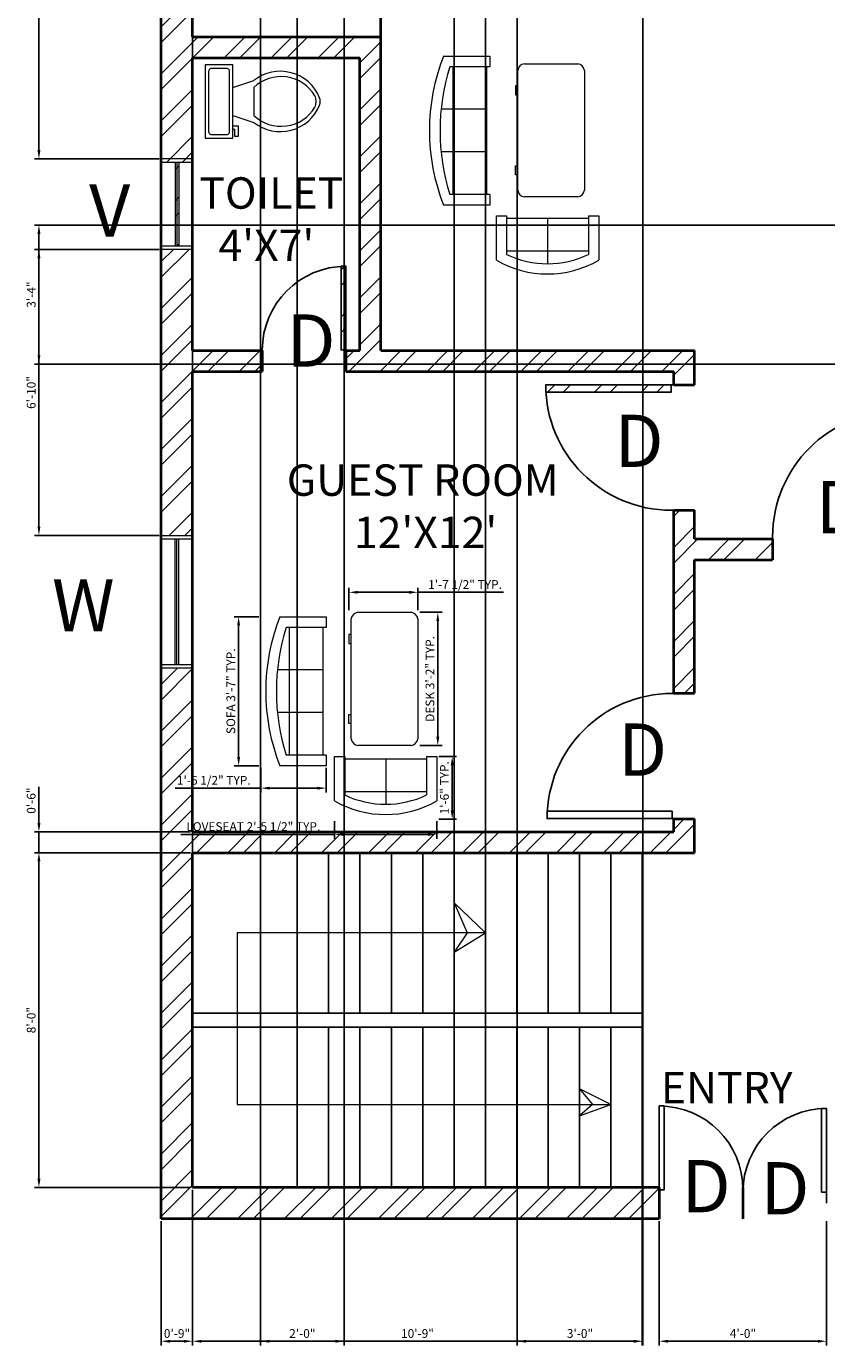
# Model space of a CAD drawing. Units: inches. Extents: x 1143 to 1626, y 7431 to 8140.
# Tile 1 of 4: x 1143 to 1373, y 7431 to 7809. Entities that reach past the tile are written whole.
import ezdxf

# ---------------------------------------------------------------- set-up
doc = ezdxf.new("R2010")
doc.units = ezdxf.units.IN
for name, color, linetype, lineweight in [('A-ANNO-DIMS', 4, 'Continuous', 18), ('A-ANNO-SYMB', 7, 'Continuous', 18), ('A-DOOR', 3, 'Continuous', 25), ('A-FLOR-STRS', 7, 'Continuous', 25), ('A-GLAZ', 4, 'Continuous', 18), ('A-WALL', 2, 'Continuous', 40), ('A-WALL-PATT', 7, 'Continuous', 13)]:
    doc.layers.add(name, color=color, linetype=linetype, lineweight=lineweight)
for name, color, linetype, lineweight, true_color in [('A-ANNO-TEXT', 40, 'Continuous', 18, 0xf8d731), ('A-AREA-IDEN', 40, 'Continuous', 25, 0xf8d731), ('A-FLOR-FIXT', 40, 'Continuous', 18, 0xf8d731), ('A-FURN', 40, 'Continuous', 18, 0xf8d731)]:
    doc.layers.add(name, color=color, linetype=linetype, lineweight=lineweight, true_color=true_color)
doc.styles.get("Standard").update_dxf_attribs({"font": 'arial.ttf'})
doc.dimstyles.new('ISO-25', dxfattribs={"dimtxt": 2.5, "dimasz": 2.5, "dimexe": 1.25, "dimexo": 0.625, "dimtad": 1, "dimdec": 0, "dimlunit": 3, "dimtxsty": 'Standard', "dimcen": 2.5, "dimadec": 0, "dimazin": 0, "dimtfac": 1, "dimtdec": 0, "dimtmove": 0, "dimatfit": 3, "dimfxl": 1, "dimarcsym": 0})

# ---------------------------------------------------------------- blocks, each defined once
blk = doc.blocks.new('*U8')
for p, q in [((0, 0), (0, -100)), ((750, 0), (750, -100))]:
    blk.add_line(p, q)
blk.add_lwpolyline([(0, 0), (0, 750), (43.75, 750), (43.75, 0)], close=True)
blk.add_arc((0, 0), 750, 0, 90)
blk = doc.blocks.new('Desk - 30 x 60 in.')
for p, q in [((-26.999995, 0), (26.999995, 0)), ((-29.999995, -27), (-29.999995, -3)), ((29.999995, -3), (29.999995, -27)), ((26.999995, -30), (-26.999995, -30)), ((-20.000005, -30), (-20.000005, -31)), ((-20.000005, -31), (-16.000005, -31)), ((-16.000005, -31), (-16.000005, -30)), ((15.999995, -31), (15.999995, -30)), ((19.999995, -31), (15.999995, -31)), ((19.999995, -30), (19.999995, -31))]:
    blk.add_line(p, q)
for centre, start, end in [((-26.499995, -3.5), 98.1301, 171.8699), ((26.499995, -3.5), 8.130102, 81.8699), ((-26.499995, -26.5), 188.1301, 261.8699), ((26.499995, -26.5), 278.1301, 351.8699)]:
    blk.add_arc(centre, 3.535534, start, end)
blk = doc.blocks.new('Sofa - Roundback 7 ft.')
for p, q in [((-12.00002, -32.4421), (-12.00003, -6.5971)), ((11.99997, -32.4421), (11.99998, -6.5971)), ((-36.000027, -34), (-36.000027, -11.4696)), ((-35.999844, -13.3819), (35.9998, -13.3819)), ((35.99998, -34), (35.99998, -11.4696)), ((-36.000027, -32.4421), (35.99998, -32.4421))]:
    blk.add_line(p, q)
for points in [[(-36.000027, -34), (-42.000027, -34), (-42.000027, -8)], [(41.99998, -8), (41.99998, -34), (35.99998, -34)]]:
    blk.add_lwpolyline(points)
for centre, radius, start, end in [((0, -114.25), 114.25, 68.43141, 111.5686), ((-0.00001, -127.1968), 121.1968, 72.72033, 107.2797)]:
    blk.add_arc(centre, radius, start, end)
blk = doc.blocks.new('Sofa - Roundback Loveseat 5 ft.')
for p, q in [((0, -32.44198), (0, -5.99998)), ((-24, -33.99998), (-24, -11.46958)), ((-23.9998, -13.38178), (23.99986, -13.38178)), ((24.00004, -33.99998), (24.00004, -11.46958)), ((-24, -32.44198), (24.00004, -32.44198))]:
    blk.add_line(p, q)
for points in [[(-24, -33.99998), (-30, -33.99998), (-30, -7.99998)], [(30.00004, -7.99998), (30.00004, -33.99998), (24.00004, -33.99998)]]:
    blk.add_lwpolyline(points)
for centre, radius, start, end in [((0, -60.24998), 60.24998, 60.13715, 119.8628), ((0, -61.38438), 55.38444, 64.32083, 115.6792)]:
    blk.add_arc(centre, radius, start, end)
blk = doc.blocks.new('Toilet - top')
for p, q in [((9.5, -6), (9.5, -2)), ((-10, -8.5), (-8, -8.5)), ((-10, -9.5), (-10, -8.5)), ((-7, -9.5), (-10, -9.5)), ((-8, -8.5), (-8, -8)), ((-7, -8), (-7, -9.5)), ((-4, -8), (-6, -14)), ((4, -8), (6, -14)), ((4, -14), (-4, -14))]:
    blk.add_line(p, q)
blk.add_lwpolyline([(10.5, -8), (10.5, 0), (-10.5, 0), (-10.5, -8)], close=True)
for points in [[(-9.5, -2), (-9.5, -6)], [(8.5, -1), (-8.5, -1)], [(-8.5, -7), (8.5, -7)]]:
    blk.add_lwpolyline(points)
for centre, radius, start, end in [((-8.62, -1.88), 0.884, 81.8699, 188.1301), ((8.62, -1.88), 0.884, 351.8699, 98.1301), ((-8.62, -6.12), 0.884, 171.8699, 278.1301), ((8.62, -6.12), 0.884, 261.8699, 8.1301), ((3.52, -21.58), 12.17, 141.4691, 247.9714), ((4.2, -21.82), 11.33, 136.3677, 238.9468), ((-3.52, -21.58), 12.17, 292.0284, 38.5307), ((-4.2, -21.82), 11.33, 301.053, 43.6321), ((0, -27.88), 4, 245.7318, 294.2682), ((0, -29), 4, 254.8605, 285.1395)]:
    blk.add_arc(centre, radius, start, end)
blk = doc.blocks.new('WIN-36IN')
for p, q in [((0, 9), (0, 0)), ((1, 9), (1, 0)), ((37, 9), (37, 0)), ((38, 9), (38, 0)), ((1, 5), (37, 5)), ((1, 4.5), (37, 4.5)), ((1, 4), (37, 4))]:
    blk.add_line(p, q)
blk = doc.blocks.new('WIN-24IN')
for p, q in [((0, 9), (0, 0)), ((1, 9), (1, 0)), ((25, 9), (25, 0)), ((26, 9), (26, 0)), ((1, 5), (25, 5)), ((1, 4.5), (25, 4.5)), ((1, 4), (25, 4))]:
    blk.add_line(p, q)
blk = doc.blocks.new('*D70')
at = {"layer": 'A-ANNO-DIMS', "color": 0, "lineweight": -2, "transparency": 16777216}
for p, q in [((1256.06, 7641.36), (1262.42, 7641.36)), ((1261.17, 7638.86), (1261.17, 7605.65)), ((1256.06, 7603.15), (1262.42, 7603.15))]:
    blk.add_line(p, q, dxfattribs=at)
at = {"layer": 'A-ANNO-DIMS', "color": 0, "transparency": 16777216}
for points in [[(1260.75, 7638.86), (1261.59, 7638.86), (1261.17, 7641.36)], [(1260.75, 7605.65), (1261.59, 7605.65), (1261.17, 7603.15)]]:
    blk.add_solid(points, dxfattribs=at)
at = {"layer": 'Defpoints', "color": 0, "transparency": 16777216}
for p in [(1255.44, 7641.36), (1255.44, 7603.15), (1261.17, 7603.15)]:
    blk.add_point(p, dxfattribs=at)
at = {"layer": 'A-ANNO-DIMS', "color": 0, "transparency": 16777216, "insert": (1259.25, 7622.25), "char_height": 2.5, "attachment_point": 5, "rotation": 90}
blk.add_mtext('DESK 3\'-2" TYP.', dxfattribs=at)
blk = doc.blocks.new('*D71')
at = {"layer": 'A-ANNO-DIMS', "color": 0, "lineweight": -2, "transparency": 16777216}
for p, q in [((1235.7, 7641.99), (1235.7, 7648.34)), ((1238.2, 7647.09), (1252.94, 7647.09)), ((1255.44, 7641.99), (1255.44, 7648.34)), ((1255.44, 7647.09), (1280.02, 7647.09))]:
    blk.add_line(p, q, dxfattribs=at)
at = {"layer": 'A-ANNO-DIMS', "color": 0, "transparency": 16777216}
for points in [[(1238.2, 7647.51), (1238.2, 7646.68), (1235.7, 7647.09)], [(1252.94, 7647.51), (1252.94, 7646.68), (1255.44, 7647.09)]]:
    blk.add_solid(points, dxfattribs=at)
at = {"layer": 'Defpoints', "color": 0, "transparency": 16777216}
for p in [(1255.44, 7647.09), (1235.7, 7641.36), (1255.44, 7641.36)]:
    blk.add_point(p, dxfattribs=at)
at = {"layer": 'A-ANNO-DIMS', "color": 0, "transparency": 16777216, "insert": (1268.98, 7649.01), "char_height": 2.5, "attachment_point": 5}
blk.add_mtext('1\'-7 1/2" TYP.', dxfattribs=at)
blk = doc.blocks.new('*D72')
at = {"layer": 'A-ANNO-DIMS', "color": 0, "lineweight": -2, "transparency": 16777216}
for p, q in [((1209.82, 7640.1), (1202.79, 7640.1)), ((1204.04, 7599.84), (1204.04, 7637.6)), ((1209.82, 7597.34), (1202.79, 7597.34))]:
    blk.add_line(p, q, dxfattribs=at)
at = {"layer": 'A-ANNO-DIMS', "color": 0, "transparency": 16777216}
for points in [[(1203.62, 7637.6), (1204.45, 7637.6), (1204.04, 7640.1)], [(1203.62, 7599.84), (1204.45, 7599.84), (1204.04, 7597.34)]]:
    blk.add_solid(points, dxfattribs=at)
at = {"layer": 'Defpoints', "color": 0, "transparency": 16777216}
for p in [(1204.04, 7640.1), (1210.45, 7640.1), (1210.45, 7597.34)]:
    blk.add_point(p, dxfattribs=at)
at = {"layer": 'A-ANNO-DIMS', "color": 0, "transparency": 16777216, "insert": (1202.12, 7618.72), "char_height": 2.5, "attachment_point": 5, "rotation": 90}
blk.add_mtext('SOFA 3\'-7" TYP.', dxfattribs=at)
blk = doc.blocks.new('*D73')
at = {"layer": 'A-ANNO-DIMS', "color": 0, "lineweight": -2, "transparency": 16777216}
for p, q in [((1210.45, 7596.72), (1210.45, 7589.68)), ((1229.11, 7596.72), (1229.11, 7589.68)), ((1210.45, 7590.93), (1185.87, 7590.93)), ((1226.61, 7590.93), (1212.95, 7590.93))]:
    blk.add_line(p, q, dxfattribs=at)
at = {"layer": 'A-ANNO-DIMS', "color": 0, "transparency": 16777216}
for points in [[(1212.95, 7591.34), (1212.95, 7590.51), (1210.45, 7590.93)], [(1226.61, 7591.34), (1226.61, 7590.51), (1229.11, 7590.93)]]:
    blk.add_solid(points, dxfattribs=at)
at = {"layer": 'Defpoints', "color": 0, "transparency": 16777216}
for p in [(1210.45, 7597.34), (1229.11, 7597.34), (1210.45, 7590.93)]:
    blk.add_point(p, dxfattribs=at)
at = {"layer": 'A-ANNO-DIMS', "color": 0, "transparency": 16777216, "insert": (1196.91, 7592.85), "char_height": 2.5, "attachment_point": 5}
blk.add_mtext('1\'-6 1/2" TYP.', dxfattribs=at)
blk = doc.blocks.new('*D74')
at = {"layer": 'A-ANNO-DIMS', "color": 0, "lineweight": -2, "transparency": 16777216}
for p, q in [((1231.54, 7581.44), (1231.54, 7576.41)), ((1260.9, 7581.44), (1260.9, 7576.41)), ((1231.54, 7577.66), (1187.43, 7577.66)), ((1258.4, 7577.66), (1234.04, 7577.66))]:
    blk.add_line(p, q, dxfattribs=at)
at = {"layer": 'A-ANNO-DIMS', "color": 0, "transparency": 16777216}
for points in [[(1234.04, 7578.07), (1234.04, 7577.24), (1231.54, 7577.66)], [(1258.4, 7578.07), (1258.4, 7577.24), (1260.9, 7577.66)]]:
    blk.add_solid(points, dxfattribs=at)
at = {"layer": 'Defpoints', "color": 0, "transparency": 16777216}
for p in [(1231.54, 7582.06), (1260.9, 7582.06), (1231.54, 7577.66)]:
    blk.add_point(p, dxfattribs=at)
at = {"layer": 'A-ANNO-DIMS', "color": 0, "transparency": 16777216, "insert": (1208.24, 7579.58), "char_height": 2.5, "attachment_point": 5}
blk.add_mtext('LOVESEAT 2\'-5 1/2" TYP.', dxfattribs=at)
blk = doc.blocks.new('*D75')
at = {"layer": 'A-ANNO-DIMS', "color": 0, "lineweight": -2, "transparency": 16777216}
for p, q in [((1261.52, 7600), (1266.55, 7600)), ((1265.3, 7597.5), (1265.3, 7584.56)), ((1261.52, 7582.06), (1266.55, 7582.06))]:
    blk.add_line(p, q, dxfattribs=at)
at = {"layer": 'A-ANNO-DIMS', "color": 0, "transparency": 16777216}
for points in [[(1264.89, 7597.5), (1265.72, 7597.5), (1265.3, 7600)], [(1264.89, 7584.56), (1265.72, 7584.56), (1265.3, 7582.06)]]:
    blk.add_solid(points, dxfattribs=at)
at = {"layer": 'Defpoints', "color": 0, "transparency": 16777216}
for p in [(1260.9, 7600), (1260.9, 7582.06), (1265.3, 7582.06)]:
    blk.add_point(p, dxfattribs=at)
at = {"layer": 'A-ANNO-DIMS', "color": 0, "transparency": 16777216, "insert": (1263.4, 7591.03), "char_height": 2.5, "attachment_point": 5, "rotation": 90}
blk.add_mtext('1\'-6" TYP.', dxfattribs=at)
blk = doc.blocks.new('*D80')
at = {"layer": 'A-ANNO-DIMS', "color": 0, "lineweight": -2, "transparency": 16777216}
for p, q in [((1190.85, 7475.77), (1190.85, 7431.05)), ((1319.85, 7475.77), (1319.85, 7431.05)), ((1193.35, 7432.3), (1317.35, 7432.3))]:
    blk.add_line(p, q, dxfattribs=at)
at = {"layer": 'A-ANNO-DIMS', "color": 0, "transparency": 16777216}
for points in [[(1193.35, 7432.71), (1193.35, 7431.88), (1190.85, 7432.3)], [(1317.35, 7432.71), (1317.35, 7431.88), (1319.85, 7432.3)]]:
    blk.add_solid(points, dxfattribs=at)
at = {"layer": 'Defpoints', "color": 0, "transparency": 16777216}
for p in [(1190.85, 7476.4), (1319.85, 7476.4), (1319.85, 7432.3)]:
    blk.add_point(p, dxfattribs=at)
at = {"layer": 'A-ANNO-DIMS', "color": 0, "transparency": 16777216, "insert": (1255.35, 7434.2), "char_height": 2.5, "attachment_point": 5}
blk.add_mtext('10\'-9"', dxfattribs=at)
blk = doc.blocks.new('*D81')
at = {"layer": 'A-ANNO-DIMS', "color": 0, "lineweight": -2, "transparency": 16777216}
for p, q in [((1190.23, 7572.4), (1145.5, 7572.4)), ((1146.75, 7478.9), (1146.75, 7569.9)), ((1190.23, 7476.4), (1145.5, 7476.4))]:
    blk.add_line(p, q, dxfattribs=at)
at = {"layer": 'A-ANNO-DIMS', "color": 0, "transparency": 16777216}
for points in [[(1146.33, 7569.9), (1147.17, 7569.9), (1146.75, 7572.4)], [(1146.33, 7478.9), (1147.17, 7478.9), (1146.75, 7476.4)]]:
    blk.add_solid(points, dxfattribs=at)
at = {"layer": 'Defpoints', "color": 0, "transparency": 16777216}
for p in [(1146.75, 7572.4), (1190.85, 7572.4), (1190.85, 7476.4)]:
    blk.add_point(p, dxfattribs=at)
at = {"layer": 'A-ANNO-DIMS', "color": 0, "transparency": 16777216, "insert": (1144.85, 7524.4), "char_height": 2.5, "attachment_point": 5, "rotation": 90}
blk.add_mtext('8\'-0"', dxfattribs=at)
blk = doc.blocks.new('*D82')
at = {"layer": 'A-ANNO-DIMS', "color": 0, "lineweight": -2, "transparency": 16777216}
for p, q in [((1324.72, 7466.77), (1324.72, 7431.05)), ((1372.72, 7466.77), (1372.72, 7431.05)), ((1327.22, 7432.3), (1370.22, 7432.3))]:
    blk.add_line(p, q, dxfattribs=at)
at = {"layer": 'A-ANNO-DIMS', "color": 0, "transparency": 16777216}
for points in [[(1327.22, 7432.71), (1327.22, 7431.88), (1324.72, 7432.3)], [(1370.22, 7432.71), (1370.22, 7431.88), (1372.72, 7432.3)]]:
    blk.add_solid(points, dxfattribs=at)
at = {"layer": 'Defpoints', "color": 0, "transparency": 16777216}
for p in [(1324.72, 7467.4), (1372.72, 7467.4), (1372.72, 7432.3)]:
    blk.add_point(p, dxfattribs=at)
at = {"layer": 'A-ANNO-DIMS', "color": 0, "transparency": 16777216, "insert": (1348.72, 7434.2), "char_height": 2.5, "attachment_point": 5}
blk.add_mtext('4\'-0"', dxfattribs=at)
blk = doc.blocks.new('*D83')
at = {"layer": 'A-ANNO-DIMS', "color": 0, "lineweight": -2, "transparency": 16777216}
for p, q in [((1190.85, 7475.77), (1190.85, 7431.05)), ((1181.85, 7466.77), (1181.85, 7431.05)), ((1184.35, 7432.3), (1188.35, 7432.3))]:
    blk.add_line(p, q, dxfattribs=at)
at = {"layer": 'A-ANNO-DIMS', "color": 0, "transparency": 16777216}
for points in [[(1184.35, 7432.71), (1184.35, 7431.88), (1181.85, 7432.3)], [(1188.35, 7432.71), (1188.35, 7431.88), (1190.85, 7432.3)]]:
    blk.add_solid(points, dxfattribs=at)
at = {"layer": 'Defpoints', "color": 0, "transparency": 16777216}
for p in [(1190.85, 7476.4), (1181.85, 7467.4), (1190.85, 7432.3)]:
    blk.add_point(p, dxfattribs=at)
at = {"layer": 'A-ANNO-DIMS', "color": 0, "transparency": 16777216, "insert": (1186.35, 7434.2), "char_height": 2.5, "attachment_point": 5}
blk.add_mtext('0\'-9"', dxfattribs=at)
blk = doc.blocks.new('*D84')
at = {"layer": 'A-ANNO-DIMS', "color": 0, "lineweight": -2, "transparency": 16777216}
for p, q in [((1146.75, 7580.9), (1146.75, 7591.29)), ((1190.23, 7578.4), (1145.5, 7578.4)), ((1146.75, 7572.4), (1146.75, 7578.4)), ((1190.23, 7572.4), (1145.5, 7572.4)), ((1146.75, 7569.9), (1146.75, 7567.4))]:
    blk.add_line(p, q, dxfattribs=at)
at = {"layer": 'A-ANNO-DIMS', "color": 0, "transparency": 16777216}
for points in [[(1146.33, 7580.9), (1147.17, 7580.9), (1146.75, 7578.4)], [(1146.33, 7569.9), (1147.17, 7569.9), (1146.75, 7572.4)]]:
    blk.add_solid(points, dxfattribs=at)
at = {"layer": 'Defpoints', "color": 0, "transparency": 16777216}
for p in [(1146.75, 7578.4), (1190.85, 7578.4), (1190.85, 7572.4)]:
    blk.add_point(p, dxfattribs=at)
at = {"layer": 'A-ANNO-DIMS', "color": 0, "transparency": 16777216, "insert": (1144.85, 7587.34), "char_height": 2.5, "attachment_point": 5, "rotation": 90}
blk.add_mtext('0\'-6"', dxfattribs=at)
blk = doc.blocks.new('*D85')
at = {"layer": 'A-ANNO-DIMS', "color": 0, "lineweight": -2, "transparency": 16777216}
for p, q in [((1283.96, 7931.77), (1283.96, 7431.05)), ((1319.96, 7931.77), (1319.96, 7431.05)), ((1286.46, 7432.3), (1317.46, 7432.3))]:
    blk.add_line(p, q, dxfattribs=at)
at = {"layer": 'A-ANNO-DIMS', "color": 0, "transparency": 16777216}
for points in [[(1286.46, 7432.71), (1286.46, 7431.88), (1283.96, 7432.3)], [(1317.46, 7432.71), (1317.46, 7431.88), (1319.96, 7432.3)]]:
    blk.add_solid(points, dxfattribs=at)
at = {"layer": 'Defpoints', "color": 0, "transparency": 16777216}
for p in [(1283.96, 7932.4), (1319.96, 7932.4), (1319.96, 7432.3)]:
    blk.add_point(p, dxfattribs=at)
at = {"layer": 'A-ANNO-DIMS', "color": 0, "transparency": 16777216, "insert": (1301.96, 7434.2), "char_height": 2.5, "attachment_point": 5}
blk.add_mtext('3\'-0"', dxfattribs=at)
blk = doc.blocks.new('*D86')
at = {"layer": 'A-ANNO-DIMS', "color": 0, "lineweight": -2, "transparency": 16777216}
for p, q in [((1210.31, 7841.77), (1210.31, 7431.05)), ((1234.31, 7841.77), (1234.31, 7431.05)), ((1212.81, 7432.3), (1231.81, 7432.3))]:
    blk.add_line(p, q, dxfattribs=at)
at = {"layer": 'A-ANNO-DIMS', "color": 0, "transparency": 16777216}
for points in [[(1212.81, 7432.71), (1212.81, 7431.88), (1210.31, 7432.3)], [(1231.81, 7432.71), (1231.81, 7431.88), (1234.31, 7432.3)]]:
    blk.add_solid(points, dxfattribs=at)
at = {"layer": 'Defpoints', "color": 0, "transparency": 16777216}
for p in [(1210.31, 7842.4), (1234.31, 7842.4), (1234.31, 7432.3)]:
    blk.add_point(p, dxfattribs=at)
at = {"layer": 'A-ANNO-DIMS', "color": 0, "transparency": 16777216, "insert": (1222.31, 7434.2), "char_height": 2.5, "attachment_point": 5}
blk.add_mtext('2\'-0"', dxfattribs=at)
blk = doc.blocks.new('*D91')
at = {"layer": 'A-ANNO-DIMS', "color": 0, "lineweight": -2, "transparency": 16777216}
for p, q in [((1181.23, 7745.4), (1145.5, 7745.4)), ((1146.75, 7665.9), (1146.75, 7742.9)), ((1181.23, 7663.4), (1145.5, 7663.4))]:
    blk.add_line(p, q, dxfattribs=at)
at = {"layer": 'A-ANNO-DIMS', "color": 0, "transparency": 16777216}
for points in [[(1146.33, 7742.9), (1147.17, 7742.9), (1146.75, 7745.4)], [(1146.33, 7665.9), (1147.17, 7665.9), (1146.75, 7663.4)]]:
    blk.add_solid(points, dxfattribs=at)
at = {"layer": 'Defpoints', "color": 0, "transparency": 16777216}
for p in [(1146.75, 7745.4), (1181.85, 7745.4), (1181.85, 7663.4)]:
    blk.add_point(p, dxfattribs=at)
at = {"layer": 'A-ANNO-DIMS', "color": 0, "transparency": 16777216, "insert": (1144.85, 7704.4), "char_height": 2.5, "attachment_point": 5, "rotation": 90}
blk.add_mtext('6\'-10"', dxfattribs=at)
blk = doc.blocks.new('*D92')
at = {"layer": 'A-ANNO-DIMS', "color": 0, "lineweight": -2, "transparency": 16777216}
for p, q in [((1181.23, 7877.4), (1145.5, 7877.4)), ((1146.75, 7773.9), (1146.75, 7874.9)), ((1181.23, 7771.4), (1145.5, 7771.4))]:
    blk.add_line(p, q, dxfattribs=at)
at = {"layer": 'A-ANNO-DIMS', "color": 0, "transparency": 16777216}
for points in [[(1146.33, 7874.9), (1147.17, 7874.9), (1146.75, 7877.4)], [(1146.33, 7773.9), (1147.17, 7773.9), (1146.75, 7771.4)]]:
    blk.add_solid(points, dxfattribs=at)
at = {"layer": 'Defpoints', "color": 0, "transparency": 16777216}
for p in [(1146.75, 7877.4), (1181.85, 7877.4), (1181.85, 7771.4)]:
    blk.add_point(p, dxfattribs=at)
at = {"layer": 'A-ANNO-DIMS', "color": 0, "transparency": 16777216, "insert": (1144.85, 7824.4), "char_height": 2.5, "attachment_point": 5, "rotation": 90}
blk.add_mtext('8\'-10"', dxfattribs=at)
blk = doc.blocks.new('*D98')
at = {"layer": 'A-ANNO-DIMS', "color": 0, "lineweight": -2, "transparency": 16777216}
for p, q in [((1190.85, 7477.02), (1190.85, 8103.75)), ((1193.35, 8102.5), (1218.35, 8102.5)), ((1220.85, 7477.02), (1220.85, 8103.75))]:
    blk.add_line(p, q, dxfattribs=at)
at = {"layer": 'A-ANNO-DIMS', "color": 0, "transparency": 16777216}
for points in [[(1193.35, 8102.91), (1193.35, 8102.08), (1190.85, 8102.5)], [(1218.35, 8102.91), (1218.35, 8102.08), (1220.85, 8102.5)]]:
    blk.add_solid(points, dxfattribs=at)
at = {"layer": 'Defpoints', "color": 0, "transparency": 16777216}
for p in [(1220.85, 8102.5), (1190.85, 7476.4), (1220.85, 7476.4)]:
    blk.add_point(p, dxfattribs=at)
at = {"layer": 'A-ANNO-DIMS', "color": 0, "transparency": 16777216, "insert": (1205.85, 8104.4), "char_height": 2.5, "attachment_point": 5}
blk.add_mtext('2\'-6"', dxfattribs=at)
blk = doc.blocks.new('*D99')
at = {"layer": 'A-ANNO-DIMS', "color": 0, "lineweight": -2, "transparency": 16777216}
for p, q in [((1265.85, 7477.02), (1265.85, 8103.75)), ((1268.35, 8102.5), (1272.35, 8102.5)), ((1274.85, 7477.02), (1274.85, 8103.75))]:
    blk.add_line(p, q, dxfattribs=at)
at = {"layer": 'A-ANNO-DIMS', "color": 0, "transparency": 16777216}
for points in [[(1268.35, 8102.91), (1268.35, 8102.08), (1265.85, 8102.5)], [(1272.35, 8102.91), (1272.35, 8102.08), (1274.85, 8102.5)]]:
    blk.add_solid(points, dxfattribs=at)
at = {"layer": 'Defpoints', "color": 0, "transparency": 16777216}
for p in [(1274.85, 8102.5), (1265.85, 7476.4), (1274.85, 7476.4)]:
    blk.add_point(p, dxfattribs=at)
at = {"layer": 'A-ANNO-DIMS', "color": 0, "transparency": 16777216, "insert": (1270.35, 8104.4), "char_height": 2.5, "attachment_point": 5}
blk.add_mtext('0\'-9"', dxfattribs=at)
blk = doc.blocks.new('*D103')
at = {"layer": 'A-ANNO-DIMS', "color": 0, "lineweight": -2, "transparency": 16777216}
for p, q in [((1430.23, 7752.4), (1145.5, 7752.4)), ((1146.75, 7715.06), (1146.75, 7749.9)), ((1430.23, 7712.56), (1145.5, 7712.56))]:
    blk.add_line(p, q, dxfattribs=at)
at = {"layer": 'A-ANNO-DIMS', "color": 0, "transparency": 16777216}
for points in [[(1146.33, 7749.9), (1147.17, 7749.9), (1146.75, 7752.4)], [(1146.33, 7715.06), (1147.17, 7715.06), (1146.75, 7712.56)]]:
    blk.add_solid(points, dxfattribs=at)
at = {"layer": 'Defpoints', "color": 0, "transparency": 16777216}
for p in [(1146.75, 7752.4), (1430.85, 7752.4), (1430.85, 7712.56)]:
    blk.add_point(p, dxfattribs=at)
at = {"layer": 'A-ANNO-DIMS', "color": 0, "transparency": 16777216, "insert": (1144.85, 7732.48), "char_height": 2.5, "attachment_point": 5, "rotation": 90}
blk.add_mtext('3\'-4"', dxfattribs=at)

msp = doc.modelspace()

# ---------------------------------------------------------------- hatches: boundary and pattern name
at = {"layer": 'A-WALL-PATT'}
h = msp.add_hatch(dxfattribs=at)
h.set_pattern_fill('ANSI32', color=256)
h.paths.add_polyline_path([(1240.85, 8067.4), (1181.85, 8067.4), (1181.85, 8017.4), (1190.85, 8017.4), (1190.85, 8058.4), (1240.85, 8058.4)])
h.paths.add_polyline_path([(1541.85, 8067.4), (1486.85, 8067.4), (1486.85, 8058.4), (1532.85, 8058.4), (1532.85, 8017.4), (1541.85, 8017.4)], flags=17)
h.paths.add_polyline_path([(1352.85, 8067.4), (1278.85, 8067.4), (1278.85, 8058.4), (1328.85, 8058.4), (1328.85, 7938.4), (1319.96, 7938.4), (1319.96, 7932.4), (1334.85, 7932.4), (1334.85, 7956.4), (1338.11, 7956.4), (1338.11, 7962.4), (1334.85, 7962.4), (1334.85, 8010.4), (1396.85, 8010.4), (1396.85, 7962.4), (1386.11, 7962.4), (1386.11, 7956.4), (1396.85, 7956.4), (1396.85, 7662.4), (1393.24, 7662.4), (1393.24, 7656.4), (1404.17, 7656.4), (1404.17, 7662.4), (1402.85, 7662.4), (1402.85, 7806.4), (1430.85, 7806.4), (1430.85, 7786.73), (1436.85, 7786.73), (1436.85, 7806.4), (1532.85, 7806.4), (1532.85, 7795.4), (1541.85, 7795.4), (1541.85, 7853.4), (1532.85, 7853.4), (1532.85, 7812.4), (1402.85, 7812.4), (1402.85, 7932.4), (1419.12, 7932.4), (1419.12, 7938.4), (1402.85, 7938.4), (1402.85, 8058.4), (1448.85, 8058.4), (1448.85, 8067.4), (1378.85, 8067.4), (1378.85, 8058.4), (1396.85, 8058.4), (1396.85, 8016.4), (1334.85, 8016.4), (1334.85, 8058.4), (1352.85, 8058.4)])
h.paths.add_polyline_path([(1283.96, 7938.4), (1190.85, 7938.4), (1190.85, 7979.4), (1181.85, 7979.4), (1181.85, 7903.4), (1190.85, 7903.4), (1190.85, 7932.4), (1238.85, 7932.4), (1238.85, 7848.4), (1234.31, 7848.4), (1234.31, 7842.4), (1244.85, 7842.4), (1244.85, 7932.4), (1283.96, 7932.4)])
h.paths.add_polyline_path([(1541.85, 7979.4), (1532.85, 7979.4), (1532.85, 7938.4), (1455.12, 7938.4), (1455.12, 7932.4), (1532.85, 7932.4), (1532.85, 7891.4), (1541.85, 7891.4)], flags=17)
h.paths.add_polyline_path([(1210.81, 7716.4), (1190.85, 7716.4), (1190.85, 7745.4), (1181.85, 7745.4), (1181.85, 7663.4), (1190.85, 7663.4), (1190.85, 7710.4), (1210.81, 7710.4)])
h.paths.add_polyline_path([(1232.89, 7871.85), (1232.89, 7871.89), (1234.29, 7871.89), (1234.29, 7847.89), (1232.89, 7847.89), (1232.89, 7871.85, 0.385662), (1210.31, 7848.85), (1210.31, 7842.4), (1190.85, 7842.4), (1190.85, 7806.4), (1244.85, 7806.4), (1244.85, 7716.4), (1325.66, 7716.4), (1334.85, 7716.4), (1334.85, 7706.63), (1328.13, 7706.63), (1328.13, 7704.53), (1292.13, 7704.53), (1292.13, 7706.63), (1328.85, 7706.63), (1328.85, 7710.4), (1325.66, 7710.4), (1234.81, 7710.4), (1234.81, 7716.6), (1233.41, 7716.6), (1233.41, 7740.6), (1234.81, 7740.6), (1234.81, 7716.4), (1238.85, 7716.4), (1238.85, 7800.4), (1190.85, 7800.4), (1190.85, 7770.4), (1186.85, 7770.4), (1186.85, 7746.4), (1185.85, 7746.4), (1185.85, 7770.4), (1181.85, 7770.4), (1181.85, 7878.4), (1190.85, 7878.4), (1190.85, 7848.4), (1210.3, 7848.4, -0.391105)])
h.paths.add_polyline_path([(1541.85, 7688.4), (1532.85, 7688.4), (1532.85, 7662.4), (1436.85, 7662.4), (1436.85, 7712.56), (1430.85, 7712.56), (1430.85, 7662.4), (1429.38, 7656.4), (1532.85, 7656.4), (1532.85, 7467.4), (1541.85, 7467.4)])
h.paths.add_polyline_path([(1334.85, 7656.4), (1357.24, 7656.4), (1357.24, 7662.4), (1334.85, 7662.4), (1334.85, 7670.63), (1328.85, 7670.63), (1328.85, 7618.14), (1334.85, 7618.14)])
h.paths.add_polyline_path([(1190.85, 7572.4), (1334.85, 7572.4), (1334.85, 7582.14), (1328.85, 7582.14), (1328.85, 7578.4), (1190.85, 7578.4), (1190.85, 7625.4), (1181.85, 7625.4), (1181.85, 7467.4), (1324.72, 7467.4), (1324.72, 7476.4), (1190.85, 7476.4)])

# ---------------------------------------------------------------- linework, layer by layer
at = {"layer": 'A-ANNO-SYMB'}
for p, q in [((1274.85, 7549.4), (1265.85, 7558.02)), ((1265.85, 7558.02), (1269.59, 7549.4)), ((1274.85, 7549.4), (1203.59, 7549.4)), ((1203.59, 7549.4), (1203.59, 7500.17)), ((1269.59, 7549.4), (1265.85, 7543.91)), ((1265.85, 7543.91), (1274.85, 7549.4)), ((1310.85, 7500.17), (1301.85, 7504.67)), ((1301.85, 7504.67), (1305.59, 7500.17)), ((1203.59, 7500.17), (1310.85, 7500.17)), ((1305.59, 7500.17), (1301.85, 7496.99)), ((1301.85, 7496.99), (1310.85, 7500.17))]:
    msp.add_line(p, q, dxfattribs=at)
at = {"layer": 'A-FLOR-STRS'}
for p, q in [((1220.85, 7476.4), (1220.85, 7572.4)), ((1229.85, 7526.4), (1229.85, 7572.4)), ((1238.85, 7526.4), (1238.85, 7572.4)), ((1247.85, 7526.4), (1247.85, 7572.4)), ((1256.85, 7526.4), (1256.85, 7572.4)), ((1265.85, 7526.4), (1265.85, 7572.4)), ((1274.85, 7526.4), (1274.85, 7572.4)), ((1283.85, 7526.4), (1283.85, 7572.4)), ((1292.85, 7526.4), (1292.85, 7572.4)), ((1301.85, 7526.4), (1301.85, 7572.4)), ((1301.85, 7526.4), (1301.85, 7572.4)), ((1310.85, 7526.4), (1310.85, 7572.4)), ((1319.85, 7476.4), (1319.85, 7572.4)), ((1319.85, 7526.4), (1190.85, 7526.4)), ((1319.85, 7522.4), (1190.85, 7522.4)), ((1229.85, 7476.4), (1229.85, 7522.4)), ((1238.85, 7476.4), (1238.85, 7522.4)), ((1247.85, 7476.4), (1247.85, 7522.4)), ((1256.85, 7476.4), (1256.85, 7522.4)), ((1265.85, 7476.4), (1265.85, 7522.4)), ((1274.85, 7476.4), (1274.85, 7522.4)), ((1283.85, 7476.4), (1283.85, 7522.4)), ((1292.85, 7476.4), (1292.85, 7522.4)), ((1301.85, 7476.4), (1301.85, 7522.4)), ((1301.85, 7476.4), (1301.85, 7522.4)), ((1310.85, 7476.4), (1310.85, 7522.4))]:
    msp.add_line(p, q, dxfattribs=at)
at = {"layer": 'A-WALL'}
for p, q in [((1181.85, 7467.4), (1181.85, 8067.4)), ((1244.85, 7716.4), (1244.85, 7932.4)), ((1190.85, 7806.4), (1190.85, 7842.4)), ((1190.85, 7806.4), (1244.85, 7806.4)), ((1190.85, 7800.4), (1238.85, 7800.4)), ((1190.85, 7716.4), (1190.85, 7800.4)), ((1238.85, 7716.4), (1238.85, 7800.4)), ((1190.85, 7716.4), (1210.81, 7716.4)), ((1210.81, 7716.4), (1210.81, 7710.4)), ((1234.81, 7716.4), (1234.81, 7710.4)), ((1234.81, 7716.4), (1238.85, 7716.4)), ((1244.85, 7716.4), (1325.66, 7716.4)), ((1325.66, 7716.4), (1334.85, 7716.4)), ((1334.85, 7706.63), (1334.85, 7716.4)), ((1190.85, 7710.4), (1210.81, 7710.4)), ((1190.85, 7578.4), (1190.85, 7710.4)), ((1234.81, 7710.4), (1325.66, 7710.4)), ((1325.66, 7710.4), (1328.85, 7710.4)), ((1328.85, 7706.63), (1328.85, 7710.4)), ((1328.85, 7706.63), (1334.85, 7706.63)), ((1328.85, 7670.63), (1334.85, 7670.63)), ((1328.85, 7618.14), (1328.85, 7670.63)), ((1334.85, 7662.4), (1334.85, 7670.63)), ((1334.85, 7662.4), (1357.24, 7662.4)), ((1357.24, 7662.4), (1357.24, 7656.4)), ((1334.85, 7656.4), (1357.24, 7656.4)), ((1334.85, 7618.14), (1334.85, 7656.4)), ((1328.85, 7618.14), (1334.85, 7618.14)), ((1328.85, 7578.4), (1328.85, 7582.14)), ((1328.85, 7582.14), (1334.85, 7582.14)), ((1334.85, 7572.4), (1334.85, 7582.14)), ((1190.85, 7578.4), (1328.85, 7578.4)), ((1190.85, 7476.4), (1190.85, 7572.4)), ((1190.85, 7572.4), (1334.85, 7572.4)), ((1324.72, 7476.4), (1190.85, 7476.4)), ((1324.72, 7476.4), (1324.72, 7467.4)), ((1348.72, 7476.4), (1348.72, 7467.4)), ((1324.72, 7467.4), (1181.85, 7467.4))]:
    msp.add_line(p, q, dxfattribs=at)

# ---------------------------------------------------------------- block references
at = {"layer": 'A-DOOR'}
for p, xscale, yscale, zscale in [((1234.81, 7716.6), -0.0320000000000001, 0.0320000000000001, 0.0320000000000001), ((1393.24, 7663), -0.0480000000000001, 0.0480000000000001, 0.0480000000000001), ((1324.72, 7475.77), 0.0320000000000002, 0.0320000000000002, 0.0320000000000002), ((1372.67, 7475.09), -0.0319465227634566, 0.0319465227634566, 0.0319465227634566)]:
    msp.add_blockref('*U8', p, dxfattribs=dict(at, xscale=xscale, yscale=yscale, zscale=zscale))
for p, xscale, yscale, zscale, rotation in [((1328.13, 7706.63), -0.0479999999999998, 0.0479999999999998, 0.0479999999999998, 90), ((1328.41, 7582.19), 0.0478464821906339, 0.0478464821906339, 0.0478464821906339, 90.00000000000003)]:
    msp.add_blockref('*U8', p, dxfattribs=dict(at, xscale=xscale, yscale=yscale, zscale=zscale, rotation=rotation))
at = {"layer": 'A-FLOR-FIXT', "rotation": 89.99999999999999}
msp.add_blockref('Toilet - top', (1194.42, 7787.86), dxfattribs=at)
at = {"layer": 'A-FURN'}
for name, p, xscale, yscale, zscale, rotation in [('Sofa - Roundback 7 ft.', (1258.77, 7779.5), 0.5089897572985498, 0.5089897572985498, 0.5089897572985498, 90), ('Desk - 30 x 60 in.', (1303.22, 7779.58), 0.6368860370765993, 0.6368860370765993, 0.6368860370765993, 270), ('Sofa - Roundback Loveseat 5 ft.', (1292.66, 7738.39), 0.4892589451312606, 0.4892589451312606, 0.4892589451312606, 180.0000000000001), ('Sofa - Roundback 7 ft.', (1211.81, 7618.72), 0.5089897572985498, 0.5089897572985498, 0.5089897572985498, 90), ('Desk - 30 x 60 in.', (1255.44, 7622.25), 0.6368860370765993, 0.6368860370765993, 0.6368860370765993, 270), ('Sofa - Roundback Loveseat 5 ft.', (1246.22, 7583.36), 0.4892589451312606, 0.4892589451312606, 0.4892589451312606, 180.0000000000001)]:
    msp.add_blockref(name, p, dxfattribs=dict(at, xscale=xscale, yscale=yscale, zscale=zscale, rotation=rotation))
at = {"layer": 'A-GLAZ'}
for name, p, rotation in [('WIN-24IN', (1181.85, 7771.4), 269.9999999999985), ('WIN-36IN', (1190.85, 7625.4), 89.99999999999692)]:
    msp.add_blockref(name, p, dxfattribs=dict(at, rotation=rotation))

# ---------------------------------------------------------------- texts
at = {"layer": 'A-ANNO-TEXT', "char_height": 15, "attachment_point": 1}
for s, insert in [('{V}', (1161.16, 7764.08)), ('{D}', (1217.75, 7726.8)), ('{D}', (1311.88, 7698.03)), ('{D}', (1369.59, 7679.04)), ('{W}', (1150.5, 7650.86)), ('{D}', (1312.87, 7609.47)), ('{D}', (1331.12, 7484.28)), ('{D}', (1353.72, 7483.66))]:
    msp.add_mtext_dynamic_manual_height_columns(s, width=1087.9578, gutter_width=12.5, heights=[0], dxfattribs=dict(at, insert=insert))
at = {"layer": 'A-AREA-IDEN', "char_height": 9, "attachment_point": 1}
for s, insert in [("{   TOILET\\P     4'X7'}", (1184.5, 7766.11)), ("{GUEST ROOM\\P       12'X12'}", (1217.86, 7683.77)), ('{ENTRY}', (1325.18, 7509.56))]:
    msp.add_mtext_dynamic_manual_height_columns(s, width=1087.9578, gutter_width=12.5, heights=[0], dxfattribs=dict(at, insert=insert))

# ---------------------------------------------------------------- dimensions: what is measured, and where the dimension line sits
at = {"layer": 'A-ANNO-DIMS'}
for base, p1, p2, picture, middle in [((1220.85, 8102.5), (1190.85, 7476.4), (1220.85, 7476.4), '*D98', (1205.85, 8104.4)), ((1274.85, 8102.5), (1265.85, 7476.4), (1274.85, 7476.4), '*D99', (1270.35, 8104.4)), ((1319.96, 7432.3), (1283.96, 7932.4), (1319.96, 7932.4), '*D85', (1301.96, 7434.2)), ((1234.31, 7432.3), (1210.31, 7842.4), (1234.31, 7842.4), '*D86', (1222.31, 7434.2)), ((1190.85, 7432.3), (1181.85, 7467.4), (1190.85, 7476.4), '*D83', (1186.35, 7434.2)), ((1319.85, 7432.3), (1190.85, 7476.4), (1319.85, 7476.4), '*D80', (1255.35, 7434.2)), ((1372.72, 7432.3), (1324.72, 7467.4), (1372.72, 7467.4), '*D82', (1348.72, 7434.2))]:
    dim = msp.add_linear_dim(base=base, p1=p1, p2=p2, dimstyle='ISO-25', override={"dimdec": 1, "dimlfac": 1, "dimrnd": 0, "dimzin": 1, "dimdsep": 46, "dimlunit": 4, "dimfrac": 2}, dxfattribs=at)
    dim.commit()
    dim.dimension.update_dxf_attribs({"geometry": picture, "text_midpoint": middle})
for base, p1, p2, picture, middle in [((1146.75, 7877.4), (1181.85, 7771.4), (1181.85, 7877.4), '*D92', (1144.85, 7824.4)), ((1146.75, 7752.4), (1430.85, 7712.56), (1430.85, 7752.4), '*D103', (1144.85, 7732.48)), ((1146.75, 7745.4), (1181.85, 7663.4), (1181.85, 7745.4), '*D91', (1144.85, 7704.4)), ((1146.75, 7578.4), (1190.85, 7572.4), (1190.85, 7578.4), '*D84', (1144.85, 7587.34)), ((1146.75, 7572.4), (1190.85, 7476.4), (1190.85, 7572.4), '*D81', (1144.85, 7524.4))]:
    dim = msp.add_linear_dim(base=base, p1=p1, p2=p2, angle=90, dimstyle='ISO-25', override={"dimdec": 1, "dimlfac": 1, "dimrnd": 0, "dimzin": 1, "dimdsep": 46, "dimlunit": 4, "dimfrac": 2}, dxfattribs=at)
    dim.commit()
    dim.dimension.update_dxf_attribs({"geometry": picture, "text_midpoint": middle})
dim = msp.add_linear_dim(base=(1255.44, 7647.09), p1=(1235.7, 7641.36), p2=(1255.44, 7641.36), text='<> TYP.', dimstyle='ISO-25', override={"dimdec": 1, "dimlfac": 1, "dimrnd": 0, "dimzin": 1, "dimdsep": 46, "dimlunit": 4, "dimfrac": 2}, dxfattribs=at)
dim.commit()
dim.dimension.update_dxf_attribs({"geometry": '*D71', "text_midpoint": (1268.98, 7649.01)})
for base, p1, p2, angle, text, picture, middle in [((1204.04, 7640.1), (1210.45, 7597.34), (1210.45, 7640.1), 90, 'SOFA <> TYP.', '*D72', (1202.12, 7618.72)), ((1261.17, 7603.15), (1255.44, 7641.36), (1255.44, 7603.15), 270, 'DESK <> TYP.', '*D70', (1259.25, 7622.25)), ((1210.45, 7590.93), (1229.11, 7597.34), (1210.45, 7597.34), 180, '<> TYP.', '*D73', (1196.91, 7592.85)), ((1265.3, 7582.06), (1260.9, 7600), (1260.9, 7582.06), 270, '<> TYP.', '*D75', (1263.4, 7591.03)), ((1231.54, 7577.66), (1260.9, 7582.06), (1231.54, 7582.06), 180, 'LOVESEAT <> TYP.', '*D74', (1208.24, 7579.58))]:
    dim = msp.add_linear_dim(base=base, p1=p1, p2=p2, angle=angle, text=text, dimstyle='ISO-25', override={"dimdec": 1, "dimlfac": 1, "dimrnd": 0, "dimzin": 1, "dimdsep": 46, "dimlunit": 4, "dimfrac": 2}, dxfattribs=at)
    dim.commit()
    dim.dimension.update_dxf_attribs({"geometry": picture, "text_midpoint": middle})

doc.saveas('drawing.dxf')
